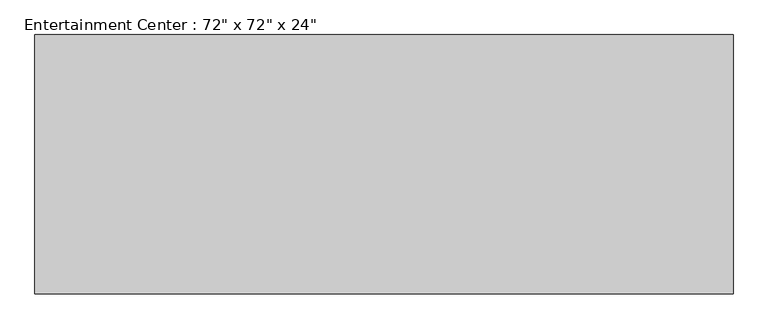
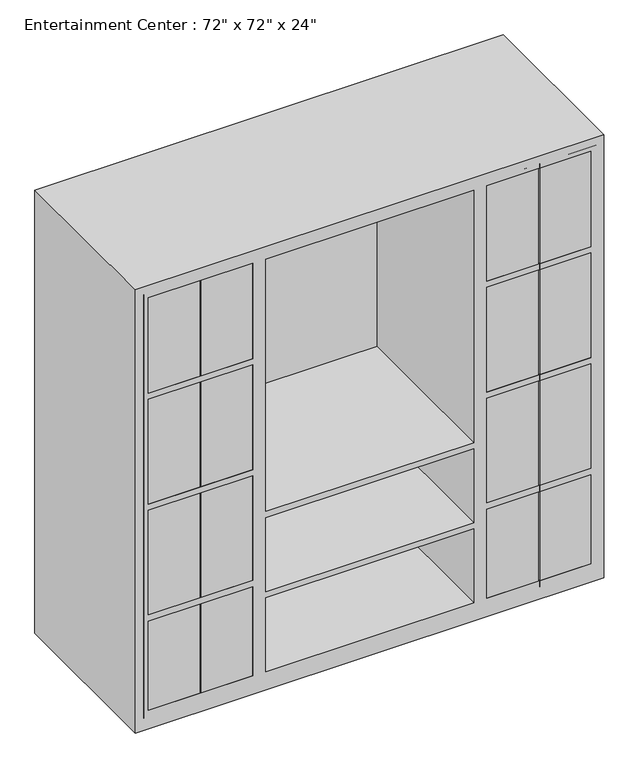
"""IFC4 building model written with IfcOpenShell, lengths in millimetres: furniture geometry."""

from ifc_helpers import new_model, si_unit, point, frame, frame_2d, origin, place, context, project, spatial, polyline, circle_curve, trimmed, segment, composite_curve, outline, extrude, faceted_brep, source, transform, mapped, element, save


def furniture_cf0b6580(model_context):
    return source(origin(), model_context, "Body", "SolidModel", [
        faceted_brep([(914.4, -781.05, 0.0), (914.4, -781.05, 1828.8), (-914.4, -781.05, 1828.8), (-914.4, -781.05, 0.0), (-457.2, -781.05, 1778.0), (-457.2, -781.05, 1384.3), (-863.6, -781.05, 1384.3), (-863.6, -781.05, 1778.0), (-457.2, -781.05, 76.2), (-863.6, -781.05, 76.2), (-863.6, -781.05, 444.5), (-457.2, -781.05, 444.5), (863.6, -781.05, 1384.3), (457.2, -781.05, 1384.3), (457.2, -781.05, 1778.0), (863.6, -781.05, 1778.0), (-406.4, -781.05, 736.6), (-406.4, -781.05, 1778.0), (406.4, -781.05, 1778.0), (406.4, -781.05, 736.6), (406.4, -781.05, 76.2), (-406.4, -781.05, 76.2), (-406.4, -781.05, 381.0), (406.4, -781.05, 381.0), (863.6, -781.05, 76.2), (457.2, -781.05, 76.2), (457.2, -781.05, 444.5), (863.6, -781.05, 444.5), (-863.6, -781.05, 469.9), (-863.6, -781.05, 901.7), (-457.2, -781.05, 901.7), (-457.2, -781.05, 469.9), (-457.2, -781.05, 1358.9), (-457.2, -781.05, 927.1), (-863.6, -781.05, 927.1), (-863.6, -781.05, 1358.9), (457.2, -781.05, 1358.9), (863.6, -781.05, 1358.9), (863.6, -781.05, 927.1), (457.2, -781.05, 927.1), (457.2, -781.05, 901.7), (863.6, -781.05, 901.7), (863.6, -781.05, 469.9), (457.2, -781.05, 469.9), (406.4, -781.05, 406.4), (-406.4, -781.05, 406.4), (-406.4, -781.05, 711.2), (406.4, -781.05, 711.2), (914.4, -101.6, 0.0), (-914.4, -101.6, 0.0), (-914.4, -101.6, 1828.8), (914.4, -101.6, 1828.8), (-457.2, -127.0, 1778.0), (-457.2, -127.0, 1384.3), (-863.6, -127.0, 1384.3), (-863.6, -127.0, 1778.0), (-457.2, -127.0, 76.2), (-863.6, -127.0, 76.2), (-863.6, -127.0, 444.5), (-457.2, -127.0, 444.5), (863.6, -127.0, 1384.3), (457.2, -127.0, 1384.3), (457.2, -127.0, 1778.0), (863.6, -127.0, 1778.0), (-406.4, -127.0, 736.6), (-406.4, -127.0, 1778.0), (406.4, -127.0, 1778.0), (406.4, -127.0, 736.6), (406.4, -127.0, 76.2), (-406.4, -127.0, 76.2), (-406.4, -127.0, 381.0), (406.4, -127.0, 381.0), (863.6, -127.0, 76.2), (457.2, -127.0, 76.2), (457.2, -127.0, 444.5), (863.6, -127.0, 444.5), (-863.6, -127.0, 469.9), (-863.6, -127.0, 901.7), (-457.2, -127.0, 901.7), (-457.2, -127.0, 469.9), (-457.2, -127.0, 1358.9), (-457.2, -127.0, 927.1), (-863.6, -127.0, 927.1), (-863.6, -127.0, 1358.9), (457.2, -127.0, 1358.9), (863.6, -127.0, 1358.9), (863.6, -127.0, 927.1), (457.2, -127.0, 927.1), (457.2, -127.0, 901.7), (863.6, -127.0, 901.7), (863.6, -127.0, 469.9), (457.2, -127.0, 469.9), (406.4, -127.0, 406.4), (-406.4, -127.0, 406.4), (-406.4, -127.0, 711.2), (406.4, -127.0, 711.2)], [[[0, 1, 2, 3], [4, 5, 6, 7], [8, 9, 10, 11], [12, 13, 14, 15], [16, 17, 18, 19], [20, 21, 22, 23], [24, 25, 26, 27], [28, 29, 30, 31], [32, 33, 34, 35], [36, 37, 38, 39], [40, 41, 42, 43], [44, 45, 46, 47]], [[48, 49, 50, 51]], [[1, 0, 48, 51]], [[2, 1, 51, 50]], [[3, 2, 50, 49]], [[0, 3, 49, 48]], [[5, 4, 52, 53]], [[6, 5, 53, 54]], [[7, 6, 54, 55]], [[4, 7, 55, 52]], [[9, 8, 56, 57]], [[10, 9, 57, 58]], [[11, 10, 58, 59]], [[8, 11, 59, 56]], [[13, 12, 60, 61]], [[14, 13, 61, 62]], [[15, 14, 62, 63]], [[12, 15, 63, 60]], [[17, 16, 64, 65]], [[18, 17, 65, 66]], [[19, 18, 66, 67]], [[16, 19, 67, 64]], [[21, 20, 68, 69]], [[22, 21, 69, 70]], [[23, 22, 70, 71]], [[20, 23, 71, 68]], [[25, 24, 72, 73]], [[26, 25, 73, 74]], [[27, 26, 74, 75]], [[24, 27, 75, 72]], [[29, 28, 76, 77]], [[30, 29, 77, 78]], [[31, 30, 78, 79]], [[28, 31, 79, 76]], [[33, 32, 80, 81]], [[34, 33, 81, 82]], [[35, 34, 82, 83]], [[32, 35, 83, 80]], [[37, 36, 84, 85]], [[38, 37, 85, 86]], [[39, 38, 86, 87]], [[36, 39, 87, 84]], [[41, 40, 88, 89]], [[42, 41, 89, 90]], [[43, 42, 90, 91]], [[40, 43, 91, 88]], [[45, 44, 92, 93]], [[46, 45, 93, 94]], [[47, 46, 94, 95]], [[44, 47, 95, 92]], [[53, 52, 55, 54]], [[57, 56, 59, 58]], [[61, 60, 63, 62]], [[65, 64, 67, 66]], [[69, 68, 71, 70]], [[73, 72, 75, 74]], [[77, 76, 79, 78]], [[81, 80, 83, 82]], [[85, 84, 87, 86]], [[89, 88, 91, 90]], [[93, 92, 95, 94]]]),
        extrude(outline(composite_curve([segment(polyline([(1003.3, -632.9986452), (1003.3, -657.225), (825.5, -657.225), (825.5, -632.9986452)]), True, "CONTINUOUS"), segment(trimmed(circle_curve(frame_2d((850.9, -632.9986452)), 25.4), [point((825.5, -632.9986452))], [point((850.9, -607.5986452))], False, "CARTESIAN"), True, "CONTINUOUS"), segment(polyline([(850.9, -607.5986452), (977.9, -607.5986452)]), True, "CONTINUOUS"), segment(trimmed(circle_curve(frame_2d((977.9, -632.9986452)), 25.4), [point((977.9, -607.5986452))], [point((1003.3, -632.9986452))], False, "CARTESIAN"), True, "CONTINUOUS")], self_intersect=False)), frame((0.0, -714.375, 0.0), z_axis=(0.0, 1.0, 0.0), x_axis=(0.0, 0.0, 1.0)), (0.0, 0.0, 1.0), 3.175),
        extrude(outline(composite_curve([segment(trimmed(circle_curve(frame_2d((977.9, -688.18125)), 25.4), [point((1003.3, -688.18125))], [point((977.9, -713.58125))], False, "CARTESIAN"), True, "CONTINUOUS"), segment(polyline([(977.9, -713.58125), (850.9, -713.58125)]), True, "CONTINUOUS"), segment(trimmed(circle_curve(frame_2d((850.9, -688.18125)), 25.4), [point((850.9, -713.58125))], [point((825.5, -688.18125))], False, "CARTESIAN"), True, "CONTINUOUS"), segment(polyline([(825.5, -688.18125), (825.5, -663.575), (1003.3, -663.575), (1003.3, -688.18125)]), True, "CONTINUOUS")], self_intersect=False)), frame((0.0, -714.375, 0.0), z_axis=(0.0, 1.0, 0.0), x_axis=(0.0, 0.0, 1.0)), (0.0, 0.0, 1.0), 3.175),
        extrude(outline(composite_curve([segment(trimmed(circle_curve(frame_2d((977.9, 632.9986452)), 25.4), [point((1003.3, 632.9986452))], [point((977.9, 607.5986452))], False, "CARTESIAN"), True, "CONTINUOUS"), segment(polyline([(977.9, 607.5986452), (850.9, 607.5986452)]), True, "CONTINUOUS"), segment(trimmed(circle_curve(frame_2d((850.9, 632.9986452)), 25.4), [point((850.9, 607.5986452))], [point((825.5, 632.9986452))], False, "CARTESIAN"), True, "CONTINUOUS"), segment(polyline([(825.5, 632.9986452), (825.5, 657.225), (1003.3, 657.225), (1003.3, 632.9986452)]), True, "CONTINUOUS")], self_intersect=False)), frame((0.0, -714.375, 0.0), z_axis=(0.0, 1.0, 0.0), x_axis=(0.0, 0.0, 1.0)), (0.0, 0.0, 1.0), 3.175),
        extrude(outline(composite_curve([segment(polyline([(1003.3, 688.18125), (1003.3, 663.575), (825.5, 663.575), (825.5, 688.18125)]), True, "CONTINUOUS"), segment(trimmed(circle_curve(frame_2d((850.9, 688.18125)), 25.4), [point((825.5, 688.18125))], [point((850.9, 713.58125))], False, "CARTESIAN"), True, "CONTINUOUS"), segment(polyline([(850.9, 713.58125), (977.9, 713.58125)]), True, "CONTINUOUS"), segment(trimmed(circle_curve(frame_2d((977.9, 688.18125)), 25.4), [point((977.9, 713.58125))], [point((1003.3, 688.18125))], False, "CARTESIAN"), True, "CONTINUOUS")], self_intersect=False)), frame((0.0, -714.375, 0.0), z_axis=(0.0, 1.0, 0.0), x_axis=(0.0, 0.0, 1.0)), (0.0, 0.0, 1.0), 3.175),
        extrude(outline(polyline([(-882.65, -711.2), (-663.575, -711.2), (-663.575, -781.05), (-882.65, -781.05), (-882.65, -711.2)])), frame((0.0, 0.0, 50.8), z_axis=(0.0, 0.0, 1.0), x_axis=(1.0, 0.0, 0.0)), (0.0, 0.0, 1.0), 1746.25),
        extrude(outline(polyline([(-657.225, -711.2), (-438.15, -711.2), (-438.15, -781.05), (-657.225, -781.05), (-657.225, -711.2)])), frame((0.0, 0.0, 50.8), z_axis=(0.0, 0.0, 1.0), x_axis=(1.0, 0.0, 0.0)), (0.0, 0.0, 1.0), 1746.25),
        extrude(outline(polyline([(663.575, -711.2), (882.65, -711.2), (882.65, -781.05), (663.575, -781.05), (663.575, -711.2)])), frame((0.0, 0.0, 50.8), z_axis=(0.0, 0.0, 1.0), x_axis=(1.0, 0.0, 0.0)), (0.0, 0.0, 1.0), 1746.25),
        extrude(outline(polyline([(438.15, -711.2), (657.225, -711.2), (657.225, -781.05), (438.15, -781.05), (438.15, -711.2)])), frame((0.0, 0.0, 50.8), z_axis=(0.0, 0.0, 1.0), x_axis=(1.0, 0.0, 0.0)), (0.0, 0.0, 1.0), 1746.25),
    ])


if __name__ == "__main__":
    model = new_model("IFC4")
    model_context = context("Model", 3, world=origin())
    ifc_project = project(units=[si_unit("LENGTHUNIT", "METRE", prefix="MILLI")], contexts=[model_context])
    site = spatial("IfcSite", under=ifc_project)
    building = spatial("IfcBuilding", under=site)
    placement = place(None, origin())
    furniture_shape = furniture_cf0b6580(model_context)
    element("IfcFurniture", 1, ObjectType="Entertainment Center : 72\" x 72\" x 24\"", at=placement, inside=building, context=model_context, shape_type="MappedRepresentation", body=[
        mapped(furniture_shape, transform((0.0, 0.0, 0.0), x_axis=(1.0, 0.0, 0.0), y_axis=(0.0, 1.0, 0.0), z_axis=(0.0, 0.0, 1.0))),
    ])
    save(model, "model.ifc")

# Revit data of these elements
# Type "Entertainment Center : 72\" x 72\" x 24\""
#   Assembly Code = "E2020200"
#   Center Width = 2' - 8"
#   Depth = 2' - 0"
#   Height = 6' - 0"
#   Width = 6' - 0"
#   Material = none
#   Default Elevation = 0
# Element 1 (IfcFurniture, "Entertainment Center : 72\" x 72\" x 24\"")
#   Materials on its faces: "Steel, Chrome Plated", "Glass - Clear, Grey"
# Materials
#   "Steel, Chrome Plated": class "Metal", colour RGB 17 17 17, transparency 0, Description = "Chromiuim plated steel", Cost = 0
#   "Glass - Clear, Grey": class "Glass", colour RGB 252 255 255, transparency 0.64
